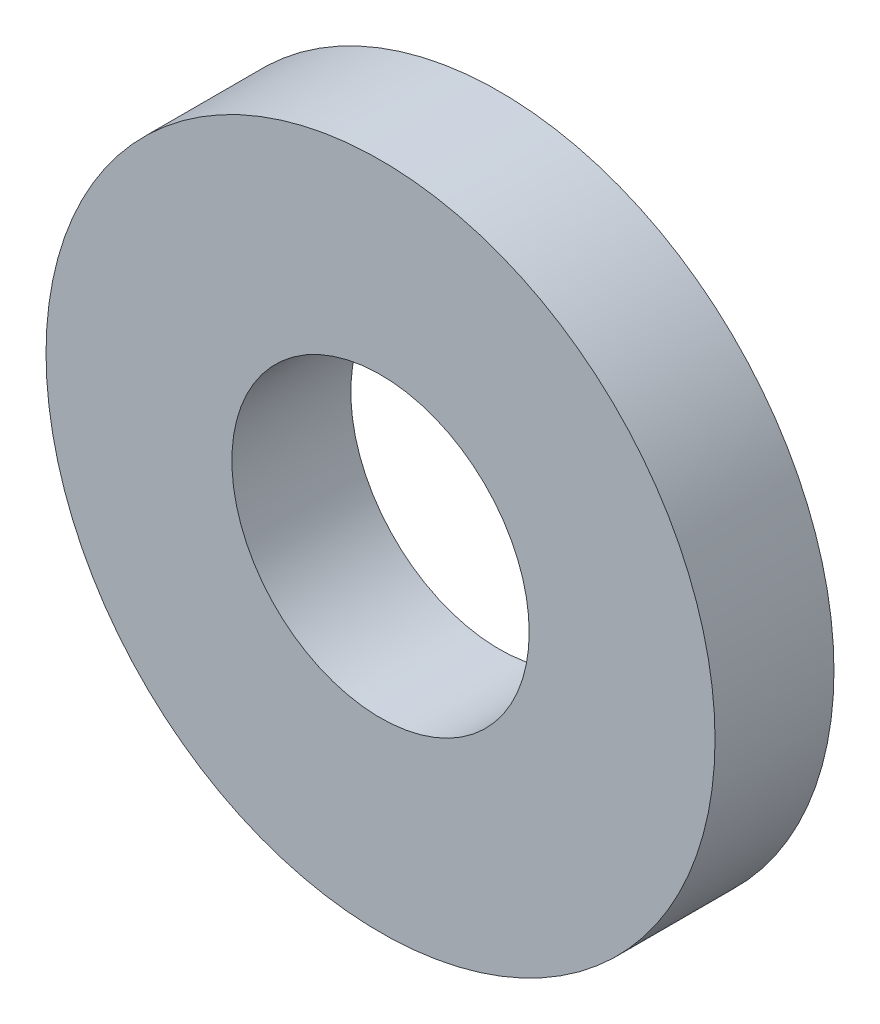
ISO-10303-21;
HEADER;
FILE_DESCRIPTION(('STEP AP214'),'2;1');
FILE_NAME('part.step','',(''),(''),'','','');
FILE_SCHEMA(('AUTOMOTIVE_DESIGN { 1 0 10303 214 1 1 1 1 }'));
ENDSEC;
DATA;
#1=APPLICATION_CONTEXT('core data for automotive mechanical design processes');
#2=APPLICATION_PROTOCOL_DEFINITION('international standard','automotive_design',2000,#1);
#3=PRODUCT_CONTEXT('',#1,'mechanical');
#4=PRODUCT('Part','Part','',(#3));
#5=PRODUCT_RELATED_PRODUCT_CATEGORY('part','',(#4));
#6=PRODUCT_DEFINITION_FORMATION('','',#4);
#7=PRODUCT_DEFINITION_CONTEXT('part definition',#1,'design');
#8=PRODUCT_DEFINITION('design','',#6,#7);
#9=PRODUCT_DEFINITION_SHAPE('','',#8);
#10=(LENGTH_UNIT() NAMED_UNIT(*) SI_UNIT(.MILLI.,.METRE.));
#11=(NAMED_UNIT(*) PLANE_ANGLE_UNIT() SI_UNIT($,.RADIAN.));
#12=(NAMED_UNIT(*) SI_UNIT($,.STERADIAN.) SOLID_ANGLE_UNIT());
#13=UNCERTAINTY_MEASURE_WITH_UNIT(LENGTH_MEASURE(1.E-05),#10,'distance_accuracy_value','');
#14=(GEOMETRIC_REPRESENTATION_CONTEXT(3) GLOBAL_UNCERTAINTY_ASSIGNED_CONTEXT((#13)) GLOBAL_UNIT_ASSIGNED_CONTEXT((#10,
#11,#12)) REPRESENTATION_CONTEXT('',''));
#15=CARTESIAN_POINT('',(0.,0.,0.));
#16=DIRECTION('',(0.,0.,1.));
#17=DIRECTION('',(1.,0.,0.));
#18=AXIS2_PLACEMENT_3D('',#15,#16,#17);
#19=CARTESIAN_POINT('',(0.,0.,8.));
#20=DIRECTION('',(0.,0.,1.));
#21=DIRECTION('',(1.,0.,0.));
#22=AXIS2_PLACEMENT_3D('',#19,#20,#21);
#23=PLANE('',#22);
#24=CARTESIAN_POINT('',(0.,0.,8.));
#25=DIRECTION('',(0.,0.,1.));
#26=DIRECTION('',(1.,0.,0.));
#27=AXIS2_PLACEMENT_3D('',#24,#25,#26);
#28=CIRCLE('',#27,22.5);
#29=CARTESIAN_POINT('',(22.5,0.,8.));
#30=VERTEX_POINT('',#29);
#31=EDGE_CURVE('E10',#30,#30,#28,.T.);
#32=ORIENTED_EDGE('',*,*,#31,.T.);
#33=EDGE_LOOP('',(#32));
#34=FACE_BOUND('',#33,.T.);
#35=CARTESIAN_POINT('',(0.,0.,8.));
#36=DIRECTION('',(0.,0.,1.));
#37=DIRECTION('',(1.,0.,0.));
#38=AXIS2_PLACEMENT_3D('',#35,#36,#37);
#39=CIRCLE('',#38,10.);
#40=CARTESIAN_POINT('',(10.,0.,8.));
#41=VERTEX_POINT('',#40);
#42=EDGE_CURVE('E48',#41,#41,#39,.T.);
#43=ORIENTED_EDGE('',*,*,#42,.F.);
#44=EDGE_LOOP('',(#43));
#45=FACE_BOUND('',#44,.T.);
#46=ADVANCED_FACE('F40',(#34,#45),#23,.T.);
#47=CARTESIAN_POINT('',(0.,0.,0.));
#48=DIRECTION('',(0.,0.,1.));
#49=DIRECTION('',(1.,0.,0.));
#50=AXIS2_PLACEMENT_3D('',#47,#48,#49);
#51=PLANE('',#50);
#52=CARTESIAN_POINT('',(0.,0.,0.));
#53=DIRECTION('',(0.,0.,1.));
#54=DIRECTION('',(1.,0.,0.));
#55=AXIS2_PLACEMENT_3D('',#52,#53,#54);
#56=CIRCLE('',#55,22.5);
#57=CARTESIAN_POINT('',(22.5,0.,0.));
#58=VERTEX_POINT('',#57);
#59=EDGE_CURVE('E41',#58,#58,#56,.T.);
#60=ORIENTED_EDGE('',*,*,#59,.F.);
#61=EDGE_LOOP('',(#60));
#62=FACE_BOUND('',#61,.T.);
#63=CARTESIAN_POINT('',(0.,0.,0.));
#64=DIRECTION('',(0.,0.,1.));
#65=DIRECTION('',(1.,0.,0.));
#66=AXIS2_PLACEMENT_3D('',#63,#64,#65);
#67=CIRCLE('',#66,10.);
#68=CARTESIAN_POINT('',(10.,0.,0.));
#69=VERTEX_POINT('',#68);
#70=EDGE_CURVE('E49',#69,#69,#67,.T.);
#71=ORIENTED_EDGE('',*,*,#70,.T.);
#72=EDGE_LOOP('',(#71));
#73=FACE_BOUND('',#72,.T.);
#74=ADVANCED_FACE('F58',(#62,#73),#51,.F.);
#75=CARTESIAN_POINT('',(0.,0.,8.));
#76=DIRECTION('',(0.,0.,-1.));
#77=DIRECTION('',(-1.,0.,0.));
#78=AXIS2_PLACEMENT_3D('',#75,#76,#77);
#79=CYLINDRICAL_SURFACE('',#78,22.5);
#80=ORIENTED_EDGE('',*,*,#31,.F.);
#81=EDGE_LOOP('',(#80));
#82=FACE_BOUND('',#81,.T.);
#83=ORIENTED_EDGE('',*,*,#59,.T.);
#84=EDGE_LOOP('',(#83));
#85=FACE_BOUND('',#84,.T.);
#86=ADVANCED_FACE('F39',(#82,#85),#79,.T.);
#87=CARTESIAN_POINT('',(0.,0.,8.));
#88=DIRECTION('',(0.,0.,-1.));
#89=DIRECTION('',(-1.,0.,0.));
#90=AXIS2_PLACEMENT_3D('',#87,#88,#89);
#91=CYLINDRICAL_SURFACE('',#90,10.);
#92=ORIENTED_EDGE('',*,*,#42,.T.);
#93=EDGE_LOOP('',(#92));
#94=FACE_BOUND('',#93,.T.);
#95=ORIENTED_EDGE('',*,*,#70,.F.);
#96=EDGE_LOOP('',(#95));
#97=FACE_BOUND('',#96,.T.);
#98=ADVANCED_FACE('F57',(#94,#97),#91,.F.);
#99=CLOSED_SHELL('',(#46,#74,#86,#98));
#100=MANIFOLD_SOLID_BREP('B2',#99);
#101=ADVANCED_BREP_SHAPE_REPRESENTATION('',(#18,#100),#14);
#102=SHAPE_DEFINITION_REPRESENTATION(#9,#101);
ENDSEC;
END-ISO-10303-21;
